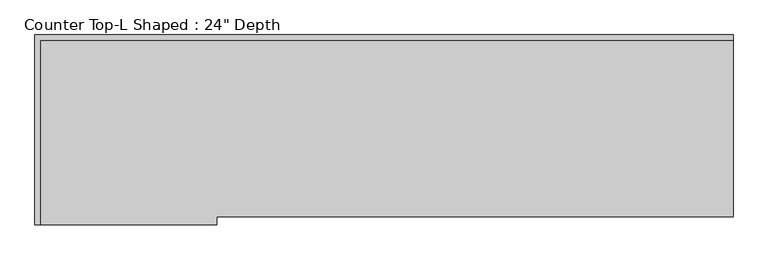
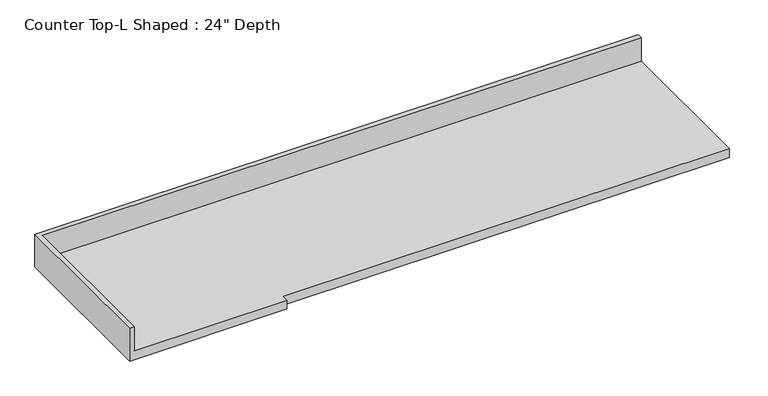
"""IFC4 building model written with IfcOpenShell, lengths in millimetres: furniture geometry."""

from ifc_helpers import new_model, si_unit, origin, place, context, project, spatial, faceted_brep, source, transform, mapped, element, save


def furniture_3ce93e2e(model_context):
    return source(origin(), model_context, "Body", "Brep", [
        faceted_brep([(-565.4622951, -662.7795346, 914.4), (-565.4622951, -635.0, 914.4), (1237.9377049, -635.0, 914.4), (1237.9377049, -19.05, 914.4), (-1181.4122951, -19.05, 914.4), (-1181.4122951, -662.7795346, 914.4), (1237.9377049, 0.0, 876.3), (1237.9377049, -635.0, 876.3), (-565.4622951, -635.0, 876.3), (-565.4622951, -662.7795346, 876.3), (-1200.4622951, -662.7795346, 876.3), (-1200.4622951, 0.0, 876.3), (-1200.4622951, 0.0, 1016.0), (1237.9377049, 0.0, 1016.0), (-1200.4622951, -662.7795346, 1016.0), (-1181.4122951, -662.7795346, 1016.0), (1237.9377049, -19.05, 1016.0), (-1181.4122951, -19.05, 1016.0)], [[[0, 1, 2, 3, 4, 5]], [[6, 7, 8, 9, 10, 11]], [[6, 11, 12, 13]], [[11, 10, 14, 12]], [[14, 10, 9, 0, 5, 15]], [[1, 0, 9, 8]], [[2, 1, 8, 7]], [[7, 6, 13, 16, 3, 2]], [[12, 14, 15, 17, 16, 13]], [[3, 16, 17, 4]], [[17, 15, 5, 4]]]),
    ])


if __name__ == "__main__":
    model = new_model("IFC4")
    model_context = context("Model", 3, world=origin())
    ifc_project = project(units=[si_unit("LENGTHUNIT", "METRE", prefix="MILLI")], contexts=[model_context])
    site = spatial("IfcSite", under=ifc_project)
    building = spatial("IfcBuilding", under=site)
    placement = place(None, origin())
    furniture_shape = furniture_3ce93e2e(model_context)
    element("IfcFurniture", 1, ObjectType="Counter Top-L Shaped : 24\" Depth", at=placement, inside=building, context=model_context, shape_type="MappedRepresentation", body=[
        mapped(furniture_shape, transform((0.0, 0.0, 0.0), x_axis=(1.0, 0.0, 0.0), y_axis=(0.0, 1.0, 0.0), z_axis=(0.0, 0.0, 1.0))),
    ])
    save(model, "model.ifc")

# Revit data of these elements
# Type "Counter Top-L Shaped : 24\" Depth"
#   Assembly Code = "C1030400"
#   Counter Thickness = 0' - 1 1/2"
#   Depth = 2' - 1"
#   Height = 3' - 0"
#   Length - Leg 1 [instance default] = 8' - 0"
#   Length - Leg 2 [instance default] = 6' - 0"
#   Counter Top Material = none
#   Default Elevation = 0
# Element 1 (IfcFurniture, "Counter Top-L Shaped : 24\" Depth")
#   Length - Leg 2 = 2' - 2.09368"
#   Materials on its faces: "Counter Top"
# Materials
#   "Counter Top": class "Wood", colour RGB 226 177 128, transparency 0
